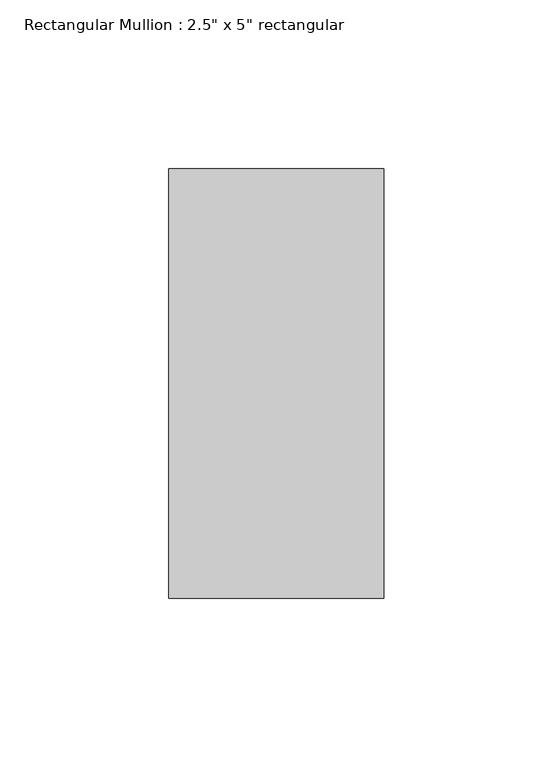
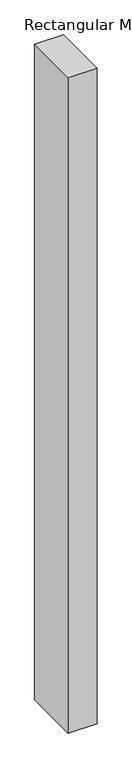
"""IFC4 building model written with IfcOpenShell, lengths in millimetres: member geometry."""

from ifc_helpers import new_model, si_unit, frame, origin, place, context, project, spatial, polyline, outline, extrude, source, transform, mapped, element, save


def member_82905deb(model_context):
    return source(origin(), model_context, "Body", "SweptSolid", [
        extrude(outline(polyline([(31.75, 63.5), (31.75, -63.5), (-31.75, -63.5), (-31.75, 63.5), (31.75, 63.5)])), frame((0.0, 0.0, -1524.0), z_axis=(0.0, 0.0, 1.0), x_axis=(1.0, 0.0, 0.0)), (0.0, 0.0, 1.0), 1524.0),
    ])


if __name__ == "__main__":
    model = new_model("IFC4")
    model_context = context("Model", 3, world=origin())
    ifc_project = project(units=[si_unit("LENGTHUNIT", "METRE", prefix="MILLI")], contexts=[model_context])
    site = spatial("IfcSite", under=ifc_project)
    building = spatial("IfcBuilding", under=site)
    placement = place(None, origin())
    member_shape = member_82905deb(model_context)
    element("IfcMember", 1, ObjectType="Rectangular Mullion : 2.5\" x 5\" rectangular", at=placement, inside=building, context=model_context, shape_type="MappedRepresentation", body=[
        mapped(member_shape, transform((0.0, 0.0, 0.0), x_axis=(1.0, 0.0, 0.0), y_axis=(0.0, 1.0, 0.0), z_axis=(0.0, 0.0, 1.0))),
    ])
    save(model, "model.ifc")

# Revit data of these elements
# Type "Rectangular Mullion : 2.5\" x 5\" rectangular"
#   built-in parameter 1007304 = 0.416667 (stored number, unit not read)
#   built-in parameter 1007301 = 0.104167 (stored number, unit not read)
#   built-in parameter 1007300 = 0.104167 (stored number, unit not read)
# Element 1 (IfcMember, "Rectangular Mullion : 2.5\" x 5\" rectangular")
#   Materials on its faces: "Aluminum"
# Materials
#   "Aluminum": class "Metal", colour RGB 247 247 247, transparency 0, Description = "Aluminum 6061", Cost = 0
